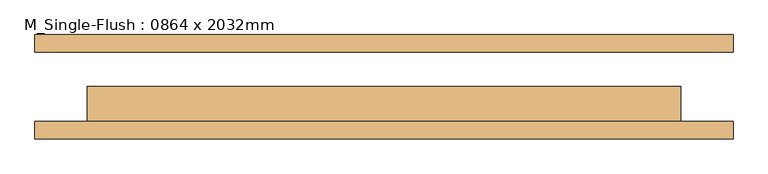
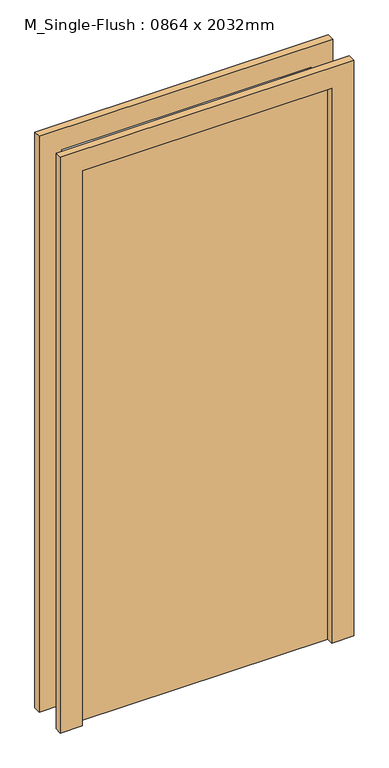
"""IFC4 building model written with IfcOpenShell, lengths in millimetres: door geometry, M_Single-Flush : 0864 x 2032mm."""

from ifc_helpers import new_model, si_unit, frame, origin, origin_with_axes, place, context, project, spatial, polyline, outline, extrude, source, transform, mapped, element, save


def m_single_flush_0864_x_2032mm_c62421c0(model_context):
    return source(origin(), model_context, "Body", "SweptSolid", [
        extrude(outline(polyline([(2108.0, -508.0), (0.0, -508.0), (0.0, -432.0), (2032.0, -432.0), (2032.0, 432.0), (0.0, 432.0), (0.0, 508.0), (2108.0, 508.0), (2108.0, -508.0)])), frame((0.0, -75.8, 0.0), z_axis=(0.0, 1.0, 0.0), x_axis=(0.0, 0.0, 1.0)), (0.0, 0.0, 1.0), 25.0),
        extrude(outline(polyline([(2108.0, 508.0), (2108.0, -508.0), (0.0, -508.0), (0.0, -432.0), (2032.0, -432.0), (2032.0, 432.0), (0.0, 432.0), (0.0, 508.0), (2108.0, 508.0)])), frame((0.0, 50.8, 0.0), z_axis=(0.0, 1.0, 0.0), x_axis=(0.0, 0.0, 1.0)), (0.0, 0.0, 1.0), 25.0),
        extrude(outline(polyline([(432.0, 0.2), (432.0, -50.8), (-432.0, -50.8), (-432.0, 0.2), (432.0, 0.2)])), origin_with_axes(), (0.0, 0.0, 1.0), 2032.0),
    ])


if __name__ == "__main__":
    model = new_model("IFC4")
    model_context = context("Model", 3, world=origin())
    ifc_project = project(units=[si_unit("LENGTHUNIT", "METRE", prefix="MILLI")], contexts=[model_context])
    site = spatial("IfcSite", under=ifc_project)
    building = spatial("IfcBuilding", under=site)
    placement = place(None, origin())
    m_single_flush_0864_x_2032mm_shape = m_single_flush_0864_x_2032mm_c62421c0(model_context)
    element("IfcDoor", 1, ObjectType="M_Single-Flush : 0864 x 2032mm", at=placement, inside=building, context=model_context, shape_type="MappedRepresentation", body=[
        mapped(m_single_flush_0864_x_2032mm_shape, transform((0.0, 0.0, 0.0), x_axis=(1.0, 0.0, 0.0), y_axis=(0.0, 1.0, 0.0), z_axis=(0.0, 0.0, 1.0))),
    ])
    save(model, "model.ifc")

# Revit data of these elements
# Type "M_Single-Flush : 0864 x 2032mm"
#   Type Mark = "32"
#   Construction Type Id = "MDOOR"
#   Analytic Construction = "Metal"
#   Thickness = 0.167323 ft
#   Thermal Resistance (R) = 0.270117 (m²·K)/W
#   Heat Transfer Coefficient (U) = 3.7021 W/(m²·K)
#   Height = 6.666667 ft
#   Trim Projection Ext = 0.082021 ft
#   Trim Projection Int = 0.082021 ft
#   Trim Width = 0.249344 ft
#   Width = 2.834646 ft
#   Define Thermal Properties by = 1
#   Define Thermal Properties by = 1
#   Door Material = Door - Panel
#   Frame Material = Door - Frame
#   Visual Light Transmittance = 0
#   Solar Heat Gain Coefficient = 0
#   Function = (empty or 0)
#   Wall Closure = (empty or 0)
# Element 1 (IfcDoor, "M_Single-Flush : 0864 x 2032mm")
#   Materials on its faces: "Door - Frame", "Door - Panel"
# Materials
#   "Door - Panel": class "Wood", colour RGB 210 159 95, transparency 0, Cost = 0
#   "Door - Frame": colour RGB 118 70 51, transparency 0, Cost = 0
